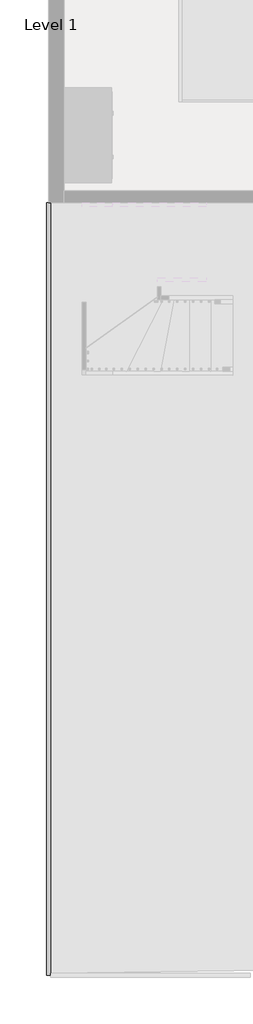
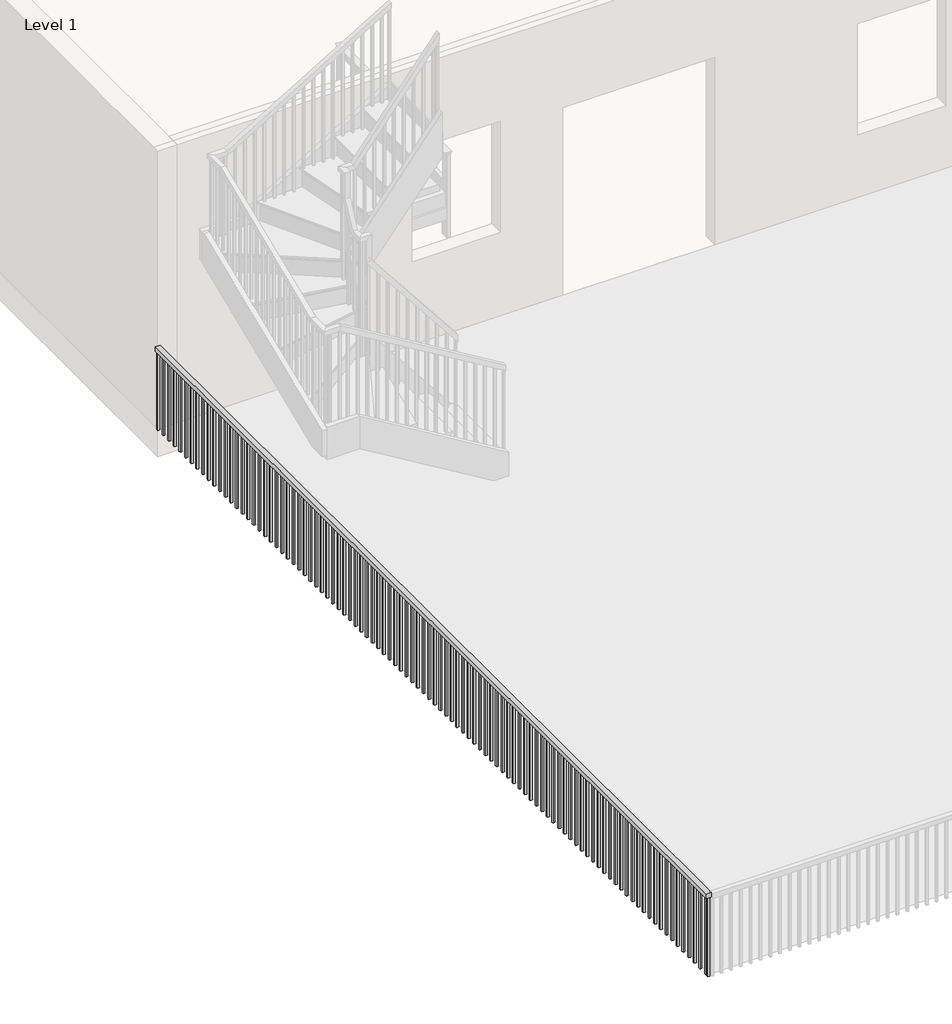
# One storey, part 2 of 5: 1 railing.
"""IFC4 building model written with IfcOpenShell, lengths in millimetres."""

from ifc_helpers import new_model, si_unit, frame, origin, origin_with_axes, place, context, project, spatial, polyline, outline, extrude, element, save

model = new_model("IFC4")

# Units and contexts
model_context = context("Model", 3, world=origin())
ifc_project = project(units=[si_unit("LENGTHUNIT", "METRE", prefix="MILLI")], contexts=[model_context])

# Site, building, storey
site = spatial("IfcSite", under=ifc_project)
building = spatial("IfcBuilding", under=site)
storey = spatial("IfcBuildingStorey", under=building, Name="Level 1", Elevation=0.0)

# Railing
placement = place(None, origin())
element("IfcRailing", 1, ObjectType="Handrail - Rectangular", at=placement, inside=storey, context=model_context, shape_type="SweptSolid", body=[
    extrude(outline(polyline([(-9037.8170266, -2473.4076646), (-8987.0170266, -2473.4076646), (-8987.0170266, -12379.4076646), (-9037.8170266, -12379.4076646), (-9037.8170266, -2473.4076646)])), frame((0.0, 0.0, 863.6), z_axis=(0.0, 0.0, 1.0), x_axis=(1.0, 0.0, 0.0)), (0.0, 0.0, 1.0), 50.8),
    extrude(outline(polyline([(-9021.9420266, -12319.0826646), (-9002.8920266, -12319.0826646), (-9002.8920266, -12338.1326646), (-9021.9420266, -12338.1326646), (-9021.9420266, -12319.0826646)])), origin_with_axes(), (0.0, 0.0, 1.0), 863.6),
    extrude(outline(polyline([(-9021.9420266, -12217.4826646), (-9002.8920266, -12217.4826646), (-9002.8920266, -12236.5326646), (-9021.9420266, -12236.5326646), (-9021.9420266, -12217.4826646)])), origin_with_axes(), (0.0, 0.0, 1.0), 863.6),
    extrude(outline(polyline([(-9021.9420266, -12115.8826646), (-9002.8920266, -12115.8826646), (-9002.8920266, -12134.9326646), (-9021.9420266, -12134.9326646), (-9021.9420266, -12115.8826646)])), origin_with_axes(), (0.0, 0.0, 1.0), 863.6),
    extrude(outline(polyline([(-9021.9420266, -12014.2826646), (-9002.8920266, -12014.2826646), (-9002.8920266, -12033.3326646), (-9021.9420266, -12033.3326646), (-9021.9420266, -12014.2826646)])), origin_with_axes(), (0.0, 0.0, 1.0), 863.6),
    extrude(outline(polyline([(-9021.9420266, -11912.6826646), (-9002.8920266, -11912.6826646), (-9002.8920266, -11931.7326646), (-9021.9420266, -11931.7326646), (-9021.9420266, -11912.6826646)])), origin_with_axes(), (0.0, 0.0, 1.0), 863.6),
    extrude(outline(polyline([(-9021.9420266, -11811.0826646), (-9002.8920266, -11811.0826646), (-9002.8920266, -11830.1326646), (-9021.9420266, -11830.1326646), (-9021.9420266, -11811.0826646)])), origin_with_axes(), (0.0, 0.0, 1.0), 863.6),
    extrude(outline(polyline([(-9021.9420266, -11709.4826646), (-9002.8920266, -11709.4826646), (-9002.8920266, -11728.5326646), (-9021.9420266, -11728.5326646), (-9021.9420266, -11709.4826646)])), origin_with_axes(), (0.0, 0.0, 1.0), 863.6),
    extrude(outline(polyline([(-9021.9420266, -11607.8826646), (-9002.8920266, -11607.8826646), (-9002.8920266, -11626.9326646), (-9021.9420266, -11626.9326646), (-9021.9420266, -11607.8826646)])), origin_with_axes(), (0.0, 0.0, 1.0), 863.6),
    extrude(outline(polyline([(-9021.9420266, -11506.2826646), (-9002.8920266, -11506.2826646), (-9002.8920266, -11525.3326646), (-9021.9420266, -11525.3326646), (-9021.9420266, -11506.2826646)])), origin_with_axes(), (0.0, 0.0, 1.0), 863.6),
    extrude(outline(polyline([(-9021.9420266, -11404.6826646), (-9002.8920266, -11404.6826646), (-9002.8920266, -11423.7326646), (-9021.9420266, -11423.7326646), (-9021.9420266, -11404.6826646)])), origin_with_axes(), (0.0, 0.0, 1.0), 863.6),
    extrude(outline(polyline([(-9021.9420266, -11303.0826646), (-9002.8920266, -11303.0826646), (-9002.8920266, -11322.1326646), (-9021.9420266, -11322.1326646), (-9021.9420266, -11303.0826646)])), origin_with_axes(), (0.0, 0.0, 1.0), 863.6),
    extrude(outline(polyline([(-9021.9420266, -11201.4826646), (-9002.8920266, -11201.4826646), (-9002.8920266, -11220.5326646), (-9021.9420266, -11220.5326646), (-9021.9420266, -11201.4826646)])), origin_with_axes(), (0.0, 0.0, 1.0), 863.6),
    extrude(outline(polyline([(-9021.9420266, -11099.8826646), (-9002.8920266, -11099.8826646), (-9002.8920266, -11118.9326646), (-9021.9420266, -11118.9326646), (-9021.9420266, -11099.8826646)])), origin_with_axes(), (0.0, 0.0, 1.0), 863.6),
    extrude(outline(polyline([(-9021.9420266, -10998.2826646), (-9002.8920266, -10998.2826646), (-9002.8920266, -11017.3326646), (-9021.9420266, -11017.3326646), (-9021.9420266, -10998.2826646)])), origin_with_axes(), (0.0, 0.0, 1.0), 863.6),
    extrude(outline(polyline([(-9021.9420266, -10896.6826646), (-9002.8920266, -10896.6826646), (-9002.8920266, -10915.7326646), (-9021.9420266, -10915.7326646), (-9021.9420266, -10896.6826646)])), origin_with_axes(), (0.0, 0.0, 1.0), 863.6),
    extrude(outline(polyline([(-9021.9420266, -10795.0826646), (-9002.8920266, -10795.0826646), (-9002.8920266, -10814.1326646), (-9021.9420266, -10814.1326646), (-9021.9420266, -10795.0826646)])), origin_with_axes(), (0.0, 0.0, 1.0), 863.6),
    extrude(outline(polyline([(-9021.9420266, -10693.4826646), (-9002.8920266, -10693.4826646), (-9002.8920266, -10712.5326646), (-9021.9420266, -10712.5326646), (-9021.9420266, -10693.4826646)])), origin_with_axes(), (0.0, 0.0, 1.0), 863.6),
    extrude(outline(polyline([(-9021.9420266, -10591.8826646), (-9002.8920266, -10591.8826646), (-9002.8920266, -10610.9326646), (-9021.9420266, -10610.9326646), (-9021.9420266, -10591.8826646)])), origin_with_axes(), (0.0, 0.0, 1.0), 863.6),
    extrude(outline(polyline([(-9021.9420266, -10490.2826646), (-9002.8920266, -10490.2826646), (-9002.8920266, -10509.3326646), (-9021.9420266, -10509.3326646), (-9021.9420266, -10490.2826646)])), origin_with_axes(), (0.0, 0.0, 1.0), 863.6),
    extrude(outline(polyline([(-9021.9420266, -10388.6826646), (-9002.8920266, -10388.6826646), (-9002.8920266, -10407.7326646), (-9021.9420266, -10407.7326646), (-9021.9420266, -10388.6826646)])), origin_with_axes(), (0.0, 0.0, 1.0), 863.6),
    extrude(outline(polyline([(-9021.9420266, -10287.0826646), (-9002.8920266, -10287.0826646), (-9002.8920266, -10306.1326646), (-9021.9420266, -10306.1326646), (-9021.9420266, -10287.0826646)])), origin_with_axes(), (0.0, 0.0, 1.0), 863.6),
    extrude(outline(polyline([(-9021.9420266, -10185.4826646), (-9002.8920266, -10185.4826646), (-9002.8920266, -10204.5326646), (-9021.9420266, -10204.5326646), (-9021.9420266, -10185.4826646)])), origin_with_axes(), (0.0, 0.0, 1.0), 863.6),
    extrude(outline(polyline([(-9021.9420266, -10083.8826646), (-9002.8920266, -10083.8826646), (-9002.8920266, -10102.9326646), (-9021.9420266, -10102.9326646), (-9021.9420266, -10083.8826646)])), origin_with_axes(), (0.0, 0.0, 1.0), 863.6),
    extrude(outline(polyline([(-9021.9420266, -9982.2826646), (-9002.8920266, -9982.2826646), (-9002.8920266, -10001.3326646), (-9021.9420266, -10001.3326646), (-9021.9420266, -9982.2826646)])), origin_with_axes(), (0.0, 0.0, 1.0), 863.6),
    extrude(outline(polyline([(-9021.9420266, -9880.6826646), (-9002.8920266, -9880.6826646), (-9002.8920266, -9899.7326646), (-9021.9420266, -9899.7326646), (-9021.9420266, -9880.6826646)])), origin_with_axes(), (0.0, 0.0, 1.0), 863.6),
    extrude(outline(polyline([(-9021.9420266, -9779.0826646), (-9002.8920266, -9779.0826646), (-9002.8920266, -9798.1326646), (-9021.9420266, -9798.1326646), (-9021.9420266, -9779.0826646)])), origin_with_axes(), (0.0, 0.0, 1.0), 863.6),
    extrude(outline(polyline([(-9021.9420266, -9677.4826646), (-9002.8920266, -9677.4826646), (-9002.8920266, -9696.5326646), (-9021.9420266, -9696.5326646), (-9021.9420266, -9677.4826646)])), origin_with_axes(), (0.0, 0.0, 1.0), 863.6),
    extrude(outline(polyline([(-9021.9420266, -9575.8826646), (-9002.8920266, -9575.8826646), (-9002.8920266, -9594.9326646), (-9021.9420266, -9594.9326646), (-9021.9420266, -9575.8826646)])), origin_with_axes(), (0.0, 0.0, 1.0), 863.6),
    extrude(outline(polyline([(-9021.9420266, -9474.2826646), (-9002.8920266, -9474.2826646), (-9002.8920266, -9493.3326646), (-9021.9420266, -9493.3326646), (-9021.9420266, -9474.2826646)])), origin_with_axes(), (0.0, 0.0, 1.0), 863.6),
    extrude(outline(polyline([(-9021.9420266, -9372.6826646), (-9002.8920266, -9372.6826646), (-9002.8920266, -9391.7326646), (-9021.9420266, -9391.7326646), (-9021.9420266, -9372.6826646)])), origin_with_axes(), (0.0, 0.0, 1.0), 863.6),
    extrude(outline(polyline([(-9021.9420266, -9271.0826646), (-9002.8920266, -9271.0826646), (-9002.8920266, -9290.1326646), (-9021.9420266, -9290.1326646), (-9021.9420266, -9271.0826646)])), origin_with_axes(), (0.0, 0.0, 1.0), 863.6),
    extrude(outline(polyline([(-9021.9420266, -9169.4826646), (-9002.8920266, -9169.4826646), (-9002.8920266, -9188.5326646), (-9021.9420266, -9188.5326646), (-9021.9420266, -9169.4826646)])), origin_with_axes(), (0.0, 0.0, 1.0), 863.6),
    extrude(outline(polyline([(-9021.9420266, -9067.8826646), (-9002.8920266, -9067.8826646), (-9002.8920266, -9086.9326646), (-9021.9420266, -9086.9326646), (-9021.9420266, -9067.8826646)])), origin_with_axes(), (0.0, 0.0, 1.0), 863.6),
    extrude(outline(polyline([(-9021.9420266, -8966.2826646), (-9002.8920266, -8966.2826646), (-9002.8920266, -8985.3326646), (-9021.9420266, -8985.3326646), (-9021.9420266, -8966.2826646)])), origin_with_axes(), (0.0, 0.0, 1.0), 863.6),
    extrude(outline(polyline([(-9021.9420266, -8864.6826646), (-9002.8920266, -8864.6826646), (-9002.8920266, -8883.7326646), (-9021.9420266, -8883.7326646), (-9021.9420266, -8864.6826646)])), origin_with_axes(), (0.0, 0.0, 1.0), 863.6),
    extrude(outline(polyline([(-9021.9420266, -8763.0826646), (-9002.8920266, -8763.0826646), (-9002.8920266, -8782.1326646), (-9021.9420266, -8782.1326646), (-9021.9420266, -8763.0826646)])), origin_with_axes(), (0.0, 0.0, 1.0), 863.6),
    extrude(outline(polyline([(-9021.9420266, -8661.4826646), (-9002.8920266, -8661.4826646), (-9002.8920266, -8680.5326646), (-9021.9420266, -8680.5326646), (-9021.9420266, -8661.4826646)])), origin_with_axes(), (0.0, 0.0, 1.0), 863.6),
    extrude(outline(polyline([(-9021.9420266, -8559.8826646), (-9002.8920266, -8559.8826646), (-9002.8920266, -8578.9326646), (-9021.9420266, -8578.9326646), (-9021.9420266, -8559.8826646)])), origin_with_axes(), (0.0, 0.0, 1.0), 863.6),
    extrude(outline(polyline([(-9021.9420266, -8458.2826646), (-9002.8920266, -8458.2826646), (-9002.8920266, -8477.3326646), (-9021.9420266, -8477.3326646), (-9021.9420266, -8458.2826646)])), origin_with_axes(), (0.0, 0.0, 1.0), 863.6),
    extrude(outline(polyline([(-9021.9420266, -8356.6826646), (-9002.8920266, -8356.6826646), (-9002.8920266, -8375.7326646), (-9021.9420266, -8375.7326646), (-9021.9420266, -8356.6826646)])), origin_with_axes(), (0.0, 0.0, 1.0), 863.6),
    extrude(outline(polyline([(-9021.9420266, -8255.0826646), (-9002.8920266, -8255.0826646), (-9002.8920266, -8274.1326646), (-9021.9420266, -8274.1326646), (-9021.9420266, -8255.0826646)])), origin_with_axes(), (0.0, 0.0, 1.0), 863.6),
    extrude(outline(polyline([(-9021.9420266, -8153.4826646), (-9002.8920266, -8153.4826646), (-9002.8920266, -8172.5326646), (-9021.9420266, -8172.5326646), (-9021.9420266, -8153.4826646)])), origin_with_axes(), (0.0, 0.0, 1.0), 863.6),
    extrude(outline(polyline([(-9021.9420266, -8051.8826646), (-9002.8920266, -8051.8826646), (-9002.8920266, -8070.9326646), (-9021.9420266, -8070.9326646), (-9021.9420266, -8051.8826646)])), origin_with_axes(), (0.0, 0.0, 1.0), 863.6),
    extrude(outline(polyline([(-9021.9420266, -7950.2826646), (-9002.8920266, -7950.2826646), (-9002.8920266, -7969.3326646), (-9021.9420266, -7969.3326646), (-9021.9420266, -7950.2826646)])), origin_with_axes(), (0.0, 0.0, 1.0), 863.6),
    extrude(outline(polyline([(-9021.9420266, -7848.6826646), (-9002.8920266, -7848.6826646), (-9002.8920266, -7867.7326646), (-9021.9420266, -7867.7326646), (-9021.9420266, -7848.6826646)])), origin_with_axes(), (0.0, 0.0, 1.0), 863.6),
    extrude(outline(polyline([(-9021.9420266, -7747.0826646), (-9002.8920266, -7747.0826646), (-9002.8920266, -7766.1326646), (-9021.9420266, -7766.1326646), (-9021.9420266, -7747.0826646)])), origin_with_axes(), (0.0, 0.0, 1.0), 863.6),
    extrude(outline(polyline([(-9021.9420266, -7645.4826646), (-9002.8920266, -7645.4826646), (-9002.8920266, -7664.5326646), (-9021.9420266, -7664.5326646), (-9021.9420266, -7645.4826646)])), origin_with_axes(), (0.0, 0.0, 1.0), 863.6),
    extrude(outline(polyline([(-9021.9420266, -7543.8826646), (-9002.8920266, -7543.8826646), (-9002.8920266, -7562.9326646), (-9021.9420266, -7562.9326646), (-9021.9420266, -7543.8826646)])), origin_with_axes(), (0.0, 0.0, 1.0), 863.6),
    extrude(outline(polyline([(-9021.9420266, -7442.2826646), (-9002.8920266, -7442.2826646), (-9002.8920266, -7461.3326646), (-9021.9420266, -7461.3326646), (-9021.9420266, -7442.2826646)])), origin_with_axes(), (0.0, 0.0, 1.0), 863.6),
    extrude(outline(polyline([(-9021.9420266, -7340.6826646), (-9002.8920266, -7340.6826646), (-9002.8920266, -7359.7326646), (-9021.9420266, -7359.7326646), (-9021.9420266, -7340.6826646)])), origin_with_axes(), (0.0, 0.0, 1.0), 863.6),
    extrude(outline(polyline([(-9021.9420266, -7239.0826646), (-9002.8920266, -7239.0826646), (-9002.8920266, -7258.1326646), (-9021.9420266, -7258.1326646), (-9021.9420266, -7239.0826646)])), origin_with_axes(), (0.0, 0.0, 1.0), 863.6),
    extrude(outline(polyline([(-9021.9420266, -7137.4826646), (-9002.8920266, -7137.4826646), (-9002.8920266, -7156.5326646), (-9021.9420266, -7156.5326646), (-9021.9420266, -7137.4826646)])), origin_with_axes(), (0.0, 0.0, 1.0), 863.6),
    extrude(outline(polyline([(-9021.9420266, -7035.8826646), (-9002.8920266, -7035.8826646), (-9002.8920266, -7054.9326646), (-9021.9420266, -7054.9326646), (-9021.9420266, -7035.8826646)])), origin_with_axes(), (0.0, 0.0, 1.0), 863.6),
    extrude(outline(polyline([(-9021.9420266, -6934.2826646), (-9002.8920266, -6934.2826646), (-9002.8920266, -6953.3326646), (-9021.9420266, -6953.3326646), (-9021.9420266, -6934.2826646)])), origin_with_axes(), (0.0, 0.0, 1.0), 863.6),
    extrude(outline(polyline([(-9021.9420266, -6832.6826646), (-9002.8920266, -6832.6826646), (-9002.8920266, -6851.7326646), (-9021.9420266, -6851.7326646), (-9021.9420266, -6832.6826646)])), origin_with_axes(), (0.0, 0.0, 1.0), 863.6),
    extrude(outline(polyline([(-9021.9420266, -6731.0826646), (-9002.8920266, -6731.0826646), (-9002.8920266, -6750.1326646), (-9021.9420266, -6750.1326646), (-9021.9420266, -6731.0826646)])), origin_with_axes(), (0.0, 0.0, 1.0), 863.6),
    extrude(outline(polyline([(-9021.9420266, -6629.4826646), (-9002.8920266, -6629.4826646), (-9002.8920266, -6648.5326646), (-9021.9420266, -6648.5326646), (-9021.9420266, -6629.4826646)])), origin_with_axes(), (0.0, 0.0, 1.0), 863.6),
    extrude(outline(polyline([(-9021.9420266, -6527.8826646), (-9002.8920266, -6527.8826646), (-9002.8920266, -6546.9326646), (-9021.9420266, -6546.9326646), (-9021.9420266, -6527.8826646)])), origin_with_axes(), (0.0, 0.0, 1.0), 863.6),
    extrude(outline(polyline([(-9021.9420266, -6426.2826646), (-9002.8920266, -6426.2826646), (-9002.8920266, -6445.3326646), (-9021.9420266, -6445.3326646), (-9021.9420266, -6426.2826646)])), origin_with_axes(), (0.0, 0.0, 1.0), 863.6),
    extrude(outline(polyline([(-9021.9420266, -6324.6826646), (-9002.8920266, -6324.6826646), (-9002.8920266, -6343.7326646), (-9021.9420266, -6343.7326646), (-9021.9420266, -6324.6826646)])), origin_with_axes(), (0.0, 0.0, 1.0), 863.6),
    extrude(outline(polyline([(-9021.9420266, -6223.0826646), (-9002.8920266, -6223.0826646), (-9002.8920266, -6242.1326646), (-9021.9420266, -6242.1326646), (-9021.9420266, -6223.0826646)])), origin_with_axes(), (0.0, 0.0, 1.0), 863.6),
    extrude(outline(polyline([(-9021.9420266, -6121.4826646), (-9002.8920266, -6121.4826646), (-9002.8920266, -6140.5326646), (-9021.9420266, -6140.5326646), (-9021.9420266, -6121.4826646)])), origin_with_axes(), (0.0, 0.0, 1.0), 863.6),
    extrude(outline(polyline([(-9021.9420266, -6019.8826646), (-9002.8920266, -6019.8826646), (-9002.8920266, -6038.9326646), (-9021.9420266, -6038.9326646), (-9021.9420266, -6019.8826646)])), origin_with_axes(), (0.0, 0.0, 1.0), 863.6),
    extrude(outline(polyline([(-9021.9420266, -5918.2826646), (-9002.8920266, -5918.2826646), (-9002.8920266, -5937.3326646), (-9021.9420266, -5937.3326646), (-9021.9420266, -5918.2826646)])), origin_with_axes(), (0.0, 0.0, 1.0), 863.6),
    extrude(outline(polyline([(-9021.9420266, -5816.6826646), (-9002.8920266, -5816.6826646), (-9002.8920266, -5835.7326646), (-9021.9420266, -5835.7326646), (-9021.9420266, -5816.6826646)])), origin_with_axes(), (0.0, 0.0, 1.0), 863.6),
    extrude(outline(polyline([(-9021.9420266, -5715.0826646), (-9002.8920266, -5715.0826646), (-9002.8920266, -5734.1326646), (-9021.9420266, -5734.1326646), (-9021.9420266, -5715.0826646)])), origin_with_axes(), (0.0, 0.0, 1.0), 863.6),
    extrude(outline(polyline([(-9021.9420266, -5613.4826646), (-9002.8920266, -5613.4826646), (-9002.8920266, -5632.5326646), (-9021.9420266, -5632.5326646), (-9021.9420266, -5613.4826646)])), origin_with_axes(), (0.0, 0.0, 1.0), 863.6),
    extrude(outline(polyline([(-9021.9420266, -5511.8826646), (-9002.8920266, -5511.8826646), (-9002.8920266, -5530.9326646), (-9021.9420266, -5530.9326646), (-9021.9420266, -5511.8826646)])), origin_with_axes(), (0.0, 0.0, 1.0), 863.6),
    extrude(outline(polyline([(-9021.9420266, -5410.2826646), (-9002.8920266, -5410.2826646), (-9002.8920266, -5429.3326646), (-9021.9420266, -5429.3326646), (-9021.9420266, -5410.2826646)])), origin_with_axes(), (0.0, 0.0, 1.0), 863.6),
    extrude(outline(polyline([(-9021.9420266, -5308.6826646), (-9002.8920266, -5308.6826646), (-9002.8920266, -5327.7326646), (-9021.9420266, -5327.7326646), (-9021.9420266, -5308.6826646)])), origin_with_axes(), (0.0, 0.0, 1.0), 863.6),
    extrude(outline(polyline([(-9021.9420266, -5207.0826646), (-9002.8920266, -5207.0826646), (-9002.8920266, -5226.1326646), (-9021.9420266, -5226.1326646), (-9021.9420266, -5207.0826646)])), origin_with_axes(), (0.0, 0.0, 1.0), 863.6),
    extrude(outline(polyline([(-9021.9420266, -5105.4826646), (-9002.8920266, -5105.4826646), (-9002.8920266, -5124.5326646), (-9021.9420266, -5124.5326646), (-9021.9420266, -5105.4826646)])), origin_with_axes(), (0.0, 0.0, 1.0), 863.6),
    extrude(outline(polyline([(-9021.9420266, -5003.8826646), (-9002.8920266, -5003.8826646), (-9002.8920266, -5022.9326646), (-9021.9420266, -5022.9326646), (-9021.9420266, -5003.8826646)])), origin_with_axes(), (0.0, 0.0, 1.0), 863.6),
    extrude(outline(polyline([(-9021.9420266, -4902.2826646), (-9002.8920266, -4902.2826646), (-9002.8920266, -4921.3326646), (-9021.9420266, -4921.3326646), (-9021.9420266, -4902.2826646)])), origin_with_axes(), (0.0, 0.0, 1.0), 863.6),
    extrude(outline(polyline([(-9021.9420266, -4800.6826646), (-9002.8920266, -4800.6826646), (-9002.8920266, -4819.7326646), (-9021.9420266, -4819.7326646), (-9021.9420266, -4800.6826646)])), origin_with_axes(), (0.0, 0.0, 1.0), 863.6),
    extrude(outline(polyline([(-9021.9420266, -4699.0826646), (-9002.8920266, -4699.0826646), (-9002.8920266, -4718.1326646), (-9021.9420266, -4718.1326646), (-9021.9420266, -4699.0826646)])), origin_with_axes(), (0.0, 0.0, 1.0), 863.6),
    extrude(outline(polyline([(-9021.9420266, -4597.4826646), (-9002.8920266, -4597.4826646), (-9002.8920266, -4616.5326646), (-9021.9420266, -4616.5326646), (-9021.9420266, -4597.4826646)])), origin_with_axes(), (0.0, 0.0, 1.0), 863.6),
    extrude(outline(polyline([(-9021.9420266, -4495.8826646), (-9002.8920266, -4495.8826646), (-9002.8920266, -4514.9326646), (-9021.9420266, -4514.9326646), (-9021.9420266, -4495.8826646)])), origin_with_axes(), (0.0, 0.0, 1.0), 863.6),
    extrude(outline(polyline([(-9021.9420266, -4394.2826646), (-9002.8920266, -4394.2826646), (-9002.8920266, -4413.3326646), (-9021.9420266, -4413.3326646), (-9021.9420266, -4394.2826646)])), origin_with_axes(), (0.0, 0.0, 1.0), 863.6),
    extrude(outline(polyline([(-9021.9420266, -4292.6826646), (-9002.8920266, -4292.6826646), (-9002.8920266, -4311.7326646), (-9021.9420266, -4311.7326646), (-9021.9420266, -4292.6826646)])), origin_with_axes(), (0.0, 0.0, 1.0), 863.6),
    extrude(outline(polyline([(-9021.9420266, -4191.0826646), (-9002.8920266, -4191.0826646), (-9002.8920266, -4210.1326646), (-9021.9420266, -4210.1326646), (-9021.9420266, -4191.0826646)])), origin_with_axes(), (0.0, 0.0, 1.0), 863.6),
    extrude(outline(polyline([(-9021.9420266, -4089.4826646), (-9002.8920266, -4089.4826646), (-9002.8920266, -4108.5326646), (-9021.9420266, -4108.5326646), (-9021.9420266, -4089.4826646)])), origin_with_axes(), (0.0, 0.0, 1.0), 863.6),
    extrude(outline(polyline([(-9021.9420266, -3987.8826646), (-9002.8920266, -3987.8826646), (-9002.8920266, -4006.9326646), (-9021.9420266, -4006.9326646), (-9021.9420266, -3987.8826646)])), origin_with_axes(), (0.0, 0.0, 1.0), 863.6),
    extrude(outline(polyline([(-9021.9420266, -3886.2826646), (-9002.8920266, -3886.2826646), (-9002.8920266, -3905.3326646), (-9021.9420266, -3905.3326646), (-9021.9420266, -3886.2826646)])), origin_with_axes(), (0.0, 0.0, 1.0), 863.6),
    extrude(outline(polyline([(-9021.9420266, -3784.6826646), (-9002.8920266, -3784.6826646), (-9002.8920266, -3803.7326646), (-9021.9420266, -3803.7326646), (-9021.9420266, -3784.6826646)])), origin_with_axes(), (0.0, 0.0, 1.0), 863.6),
    extrude(outline(polyline([(-9021.9420266, -3683.0826646), (-9002.8920266, -3683.0826646), (-9002.8920266, -3702.1326646), (-9021.9420266, -3702.1326646), (-9021.9420266, -3683.0826646)])), origin_with_axes(), (0.0, 0.0, 1.0), 863.6),
    extrude(outline(polyline([(-9021.9420266, -3581.4826646), (-9002.8920266, -3581.4826646), (-9002.8920266, -3600.5326646), (-9021.9420266, -3600.5326646), (-9021.9420266, -3581.4826646)])), origin_with_axes(), (0.0, 0.0, 1.0), 863.6),
    extrude(outline(polyline([(-9021.9420266, -3479.8826646), (-9002.8920266, -3479.8826646), (-9002.8920266, -3498.9326646), (-9021.9420266, -3498.9326646), (-9021.9420266, -3479.8826646)])), origin_with_axes(), (0.0, 0.0, 1.0), 863.6),
    extrude(outline(polyline([(-9021.9420266, -3378.2826646), (-9002.8920266, -3378.2826646), (-9002.8920266, -3397.3326646), (-9021.9420266, -3397.3326646), (-9021.9420266, -3378.2826646)])), origin_with_axes(), (0.0, 0.0, 1.0), 863.6),
    extrude(outline(polyline([(-9021.9420266, -3276.6826646), (-9002.8920266, -3276.6826646), (-9002.8920266, -3295.7326646), (-9021.9420266, -3295.7326646), (-9021.9420266, -3276.6826646)])), origin_with_axes(), (0.0, 0.0, 1.0), 863.6),
    extrude(outline(polyline([(-9021.9420266, -3175.0826646), (-9002.8920266, -3175.0826646), (-9002.8920266, -3194.1326646), (-9021.9420266, -3194.1326646), (-9021.9420266, -3175.0826646)])), origin_with_axes(), (0.0, 0.0, 1.0), 863.6),
    extrude(outline(polyline([(-9021.9420266, -3073.4826646), (-9002.8920266, -3073.4826646), (-9002.8920266, -3092.5326646), (-9021.9420266, -3092.5326646), (-9021.9420266, -3073.4826646)])), origin_with_axes(), (0.0, 0.0, 1.0), 863.6),
    extrude(outline(polyline([(-9021.9420266, -2971.8826646), (-9002.8920266, -2971.8826646), (-9002.8920266, -2990.9326646), (-9021.9420266, -2990.9326646), (-9021.9420266, -2971.8826646)])), origin_with_axes(), (0.0, 0.0, 1.0), 863.6),
    extrude(outline(polyline([(-9021.9420266, -2870.2826646), (-9002.8920266, -2870.2826646), (-9002.8920266, -2889.3326646), (-9021.9420266, -2889.3326646), (-9021.9420266, -2870.2826646)])), origin_with_axes(), (0.0, 0.0, 1.0), 863.6),
    extrude(outline(polyline([(-9021.9420266, -2768.6826646), (-9002.8920266, -2768.6826646), (-9002.8920266, -2787.7326646), (-9021.9420266, -2787.7326646), (-9021.9420266, -2768.6826646)])), origin_with_axes(), (0.0, 0.0, 1.0), 863.6),
    extrude(outline(polyline([(-9021.9420266, -2667.0826646), (-9002.8920266, -2667.0826646), (-9002.8920266, -2686.1326646), (-9021.9420266, -2686.1326646), (-9021.9420266, -2667.0826646)])), origin_with_axes(), (0.0, 0.0, 1.0), 863.6),
    extrude(outline(polyline([(-9021.9420266, -2565.4826646), (-9002.8920266, -2565.4826646), (-9002.8920266, -2584.5326646), (-9021.9420266, -2584.5326646), (-9021.9420266, -2565.4826646)])), origin_with_axes(), (0.0, 0.0, 1.0), 863.6),
    extrude(outline(polyline([(-9021.9420266, -12360.3576646), (-9002.8920266, -12360.3576646), (-9002.8920266, -12379.4076646), (-9021.9420266, -12379.4076646), (-9021.9420266, -12360.3576646)])), origin_with_axes(), (0.0, 0.0, 1.0), 863.6),
    extrude(outline(polyline([(-9021.9420266, -2473.4076646), (-9002.8920266, -2473.4076646), (-9002.8920266, -2492.4576646), (-9021.9420266, -2492.4576646), (-9021.9420266, -2473.4076646)])), origin_with_axes(), (0.0, 0.0, 1.0), 863.6),
])

save(model, "model.ifc")

# Revit data of these elements
# Type "Handrail - Rectangular"
#   Assembly Code = "C2010400"
#   built-in parameter 1008612 = 0.0416667 (stored number, unit not read)
#   built-in parameter 1008611 = 0.0416667 (stored number, unit not read)
#   built-in parameter 1008609 = 0.333333 (stored number, unit not read)
#   built-in parameter 1008604 = 0.166667 (stored number, unit not read)
#   built-in parameter 1008603 = 0.166667 (stored number, unit not read)
#   Railing Height = 3' - 0"
#   built-in parameter 1008630 = 2
#   built-in parameter 1008610 = 2
#   built-in parameter 1008618 = Baluster - Square : 3/4"
# Element 1 (IfcRailing, "Handrail - Rectangular")
#   Phase Created = New Construction
